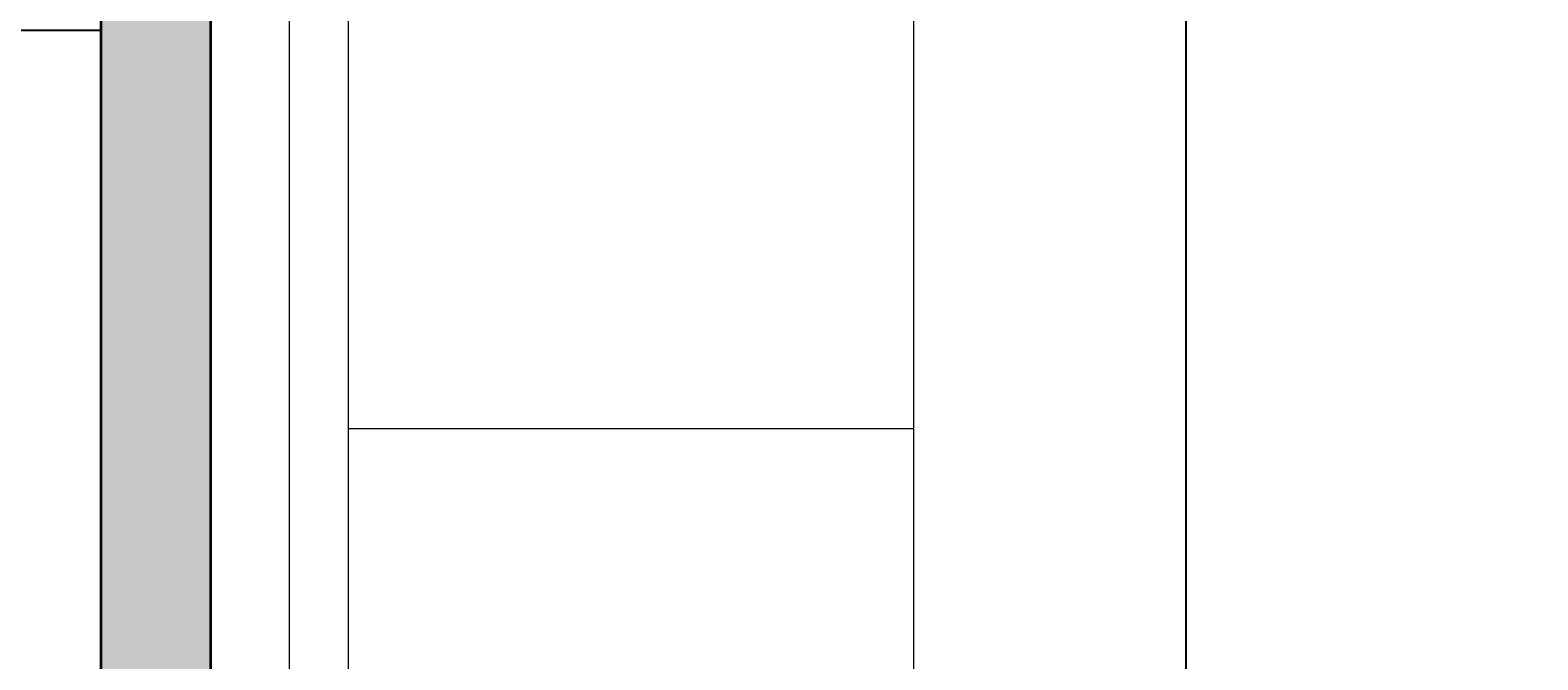
# Model space of a CAD drawing. Units: inches. Extents: x 1998 to 2588, y 1139 to 1977.
# Tile 47 of 134: x 2220 to 2282, y 1637 to 1663. Entities that reach past the tile are written whole.
import ezdxf

# ---------------------------------------------------------------- set-up
doc = ezdxf.new("R2010")
doc.units = ezdxf.units.IN
for name, color, linetype, lineweight in [('A-ANNO-DIMS', 2, 'Continuous', 18), ('A-FLOR-CASE', 32, 'Continuous', 25), ('A-WALL-PATT', 252, 'Continuous', 13), ('FUR', 21, 'Continuous', 18), ('WALL', 200, 'Continuous', 35)]:
    doc.layers.add(name, color=color, linetype=linetype, lineweight=lineweight)
doc.styles.get("Standard").update_dxf_attribs({"font": 'arial.ttf'})
doc.dimstyles.get("Standard").update_dxf_attribs({"dimtxt": 0.18, "dimasz": 0.18, "dimexe": 0.18, "dimexo": 0.0625, "dimgap": 0.09, "dimtad": 0, "dimtih": 1, "dimtoh": 1, "dimdec": 4, "dimzin": 0, "dimdsep": 46, "dimtxsty": 'Standard', "dimcen": 0.09, "dimadec": 0, "dimazin": 0, "dimtfac": 1, "dimtdec": 4, "dimtofl": 0, "dimtmove": 0, "dimatfit": 3, "dimfxl": 1, "dimtolj": 1, "dimtzin": 0, "dimarcsym": 0})

# ---------------------------------------------------------------- blocks, each defined once
blk = doc.blocks.new('SOFA-THREE-SEAT')
for p, q in [((24.453, 25.615), (24.453, 2.416)), ((0, 0), (74.336, 0))]:
    blk.add_line(p, q)
blk.add_lwpolyline([(3.604, 2.416), (71.008, 2.416), (71.008, 25.615), (3.604, 25.615)], close=True)
blk = doc.blocks.new('*D11')
at = {"layer": 'A-ANNO-DIMS', "color": 0, "lineweight": -2, "transparency": 16777216}
for p, q in [((2256.378, 1671.356), (2267.646, 1671.356)), ((2267.466, 1671.176), (2267.466, 1634.372)), ((2267.466, 1597.201), (2267.466, 1634.005)), ((2256.378, 1597.021), (2267.646, 1597.021))]:
    blk.add_line(p, q, dxfattribs=at)
at = {"layer": 'A-ANNO-DIMS', "color": 0, "transparency": 16777216}
for points in [[(2267.436, 1671.176), (2267.496, 1671.176), (2267.466, 1671.356)], [(2267.436, 1597.201), (2267.496, 1597.201), (2267.466, 1597.021)]]:
    blk.add_solid(points, dxfattribs=at)
at = {"layer": 'Defpoints', "color": 0, "transparency": 16777216}
for p in [(2256.316, 1671.356), (2256.316, 1597.021), (2267.466, 1597.021)]:
    blk.add_point(p, dxfattribs=at)
at = {"layer": 'A-ANNO-DIMS', "color": 0, "transparency": 16777216, "insert": (2267.466, 1634.189), "char_height": 0.18, "attachment_point": 5}
blk.add_mtext('\\A1;SOFA 74 TYP.', dxfattribs=at)

msp = doc.modelspace()

# ---------------------------------------------------------------- hatches: boundary and pattern name
at = {"layer": 'A-WALL-PATT'}
h = msp.add_hatch(color=256, dxfattribs=at)
h.dxf.hatch_style = 1
h.paths.add_polyline_path([(2527.4729, 1362.2324), (2510.9729, 1362.2324), (2510.9729, 1357.7324), (2518.4729, 1357.7324), (2518.4729, 1237.7324), (2503.1458, 1237.7324), (2503.1458, 1228.7324), (2527.4729, 1228.7324)])
h.paths.add_polyline_path([(2490.5682, 1362.2324), (2398.4729, 1362.2324), (2398.4729, 1357.7324), (2490.5682, 1357.7324)])
h.paths.add_polyline_path([(2224.9729, 1264.7324), (2222.9729, 1264.7324), (2222.9729, 1232.4125), (2341.4729, 1232.4125), (2341.4729, 1234.4125), (2224.9729, 1234.4125)])
h.paths.add_polyline_path([(2334.5332, 1273.7324), (2264.7638, 1273.7324), (2264.7638, 1269.5611, -0.043659), (2264.3413, 1264.7324), (2334.5332, 1264.7324)])
h.paths.add_polyline_path([(2236.9551, 1273.7324), (2234.4125, 1273.7324), (2234.4125, 1264.7324), (2236.9551, 1264.7324), (2236.9551, 1269.5611)])
h.paths.add_polyline_path([(2222.9729, 1293.2324), (2096.9729, 1293.2324), (2096.9729, 1345.0966), (2087.9729, 1345.0966), (2087.9729, 1284.2324), (2222.9729, 1284.2324), (2222.9729, 1285.137)])
h.paths.add_polyline_path([(2096.9729, 1458.7927), (2087.9729, 1458.7927), (2087.9729, 1417.7324), (2087.9729, 1413.2324), (2096.9729, 1413.2324), (2096.9729, 1417.7324)])
h.paths.add_polyline_path([(2096.9729, 1413.2324), (2087.9729, 1413.2324), (2087.9729, 1365.5012), (2096.9729, 1365.5012), (2096.9729, 1369.3358)])
h.paths.add_polyline_path([(2186.2943, 1417.7324), (2138.6074, 1417.7324), (2096.9729, 1417.7324), (2096.9729, 1413.2324), (2138.6074, 1413.2324), (2186.2943, 1413.2324)])
h.paths.add_polyline_path([(2181.4729, 1465.7324), (2176.9729, 1465.7324), (2176.9729, 1451.6434), (2181.4729, 1451.6434)])
h.paths.add_polyline_path([(2181.4729, 1422.1664), (2176.9729, 1422.1664), (2176.9729, 1417.7324), (2181.4729, 1417.7324)])
h.paths.add_polyline_path([(2063.9729, 1465.7324), (2087.9729, 1465.7324), (2087.9729, 1470.2324), (2059.4729, 1470.2324), (2059.4729, 1413.2324), (2087.9729, 1413.2324), (2087.9729, 1417.7324), (2063.9729, 1417.7324)])
h.paths.add_polyline_path([(2181.4729, 1755.2324), (2176.9729, 1755.2324), (2176.9729, 1748.6798), (2177.0513, 1748.6798), (2181.4729, 1748.6798)])
h.paths.add_polyline_path([(2227.4729, 1707.2324), (2220.4647, 1707.2324), (2220.4647, 1702.7324), (2222.9729, 1702.7324), (2222.9729, 1604.637), (2227.4729, 1604.637)])
h.paths.add_polyline_path([(2114.9729, 1702.7324), (2105.9729, 1702.7324), (2105.9729, 1628.4781, -0.0318759), (2110.1012, 1628.7416), (2114.9729, 1628.7416)])
h.paths.add_polyline_path([(2345.9729, 1739.3278), (2341.4729, 1739.3278), (2341.4729, 1647.5211), (2345.9729, 1647.5211)])
h.paths.add_polyline_path([(2350.6273, 1641.2324), (2345.9729, 1641.2324), (2345.9729, 1636.7324), (2350.6273, 1636.7324), (2350.6273, 1639.8729)])
h.paths.add_polyline_path([(2501.9729, 1641.2324), (2407.9729, 1641.2324), (2392.5005, 1641.2324), (2392.5005, 1639.8729), (2392.5005, 1636.7324), (2501.9729, 1636.7324)])
h.paths.add_polyline_path([(2510.9729, 1755.2324), (2501.9729, 1755.2324), (2501.9729, 1641.2324), (2510.9729, 1641.2324)])
h.paths.add_polyline_path([(2549.1786, 1641.2324), (2522.3775, 1641.2324), (2522.3775, 1636.7324), (2540.1786, 1636.7324), (2540.1786, 1480.7324), (2522.3775, 1480.7324), (2522.3775, 1476.2324), (2549.1786, 1476.2324)])
h.paths.add_polyline_path([(2498.1786, 1594.7324), (2407.9729, 1594.7324), (2407.9729, 1585.7324), (2416.9729, 1585.7324), (2489.1786, 1585.7324), (2489.1786, 1531.7324), (2416.9729, 1531.7324), (2407.9729, 1531.7324), (2407.9729, 1522.7324), (2498.1786, 1522.7324)])
h.paths.add_polyline_path([(2351.6437, 1480.7324), (2345.9729, 1480.7324), (2345.9729, 1476.2324), (2351.6437, 1476.2324), (2351.6437, 1477.5919)])
h.paths.add_polyline_path([(2501.9729, 1480.7324), (2498.1786, 1480.7324), (2407.9729, 1480.7324), (2393.5168, 1480.7324), (2393.5168, 1477.5919), (2393.5168, 1476.2324), (2501.9729, 1476.2324)])

# ---------------------------------------------------------------- linework, layer by layer
at = {"layer": 'A-FLOR-CASE'}
msp.add_line((2197.4499, 1663.2466), (2222.9729, 1663.2466), dxfattribs=at)
at = {"layer": 'WALL'}
for p, q in [((2227.4729, 1707.2324), (2227.4729, 1584.2324)), ((2222.9729, 1702.7324), (2222.9729, 1604.637))]:
    msp.add_line(p, q, dxfattribs=at)

# ---------------------------------------------------------------- block references
at = {"layer": 'FUR', "rotation": 270.0000000000001}
msp.add_blockref('SOFA-THREE-SEAT', (2230.701, 1671.3567), dxfattribs=at)

# ---------------------------------------------------------------- dimensions: what is measured, and where the dimension line sits
at = {"layer": 'A-ANNO-DIMS'}
dim = msp.add_linear_dim(base=(2267.4662, 1597.0205), p1=(2256.3158, 1671.3565), p2=(2256.3158, 1597.0205), angle=270, text='SOFA <> TYP.', dimstyle='Standard', override={"dimdec": 0, "dimlfac": 1, "dimrnd": 0, "dimzin": 0, "dimdsep": 46, "dimlunit": 2}, dxfattribs=at)
dim.commit()
dim.dimension.update_dxf_attribs({"geometry": '*D11', "text_midpoint": (2267.4662, 1634.1885)})

doc.saveas('drawing.dxf')
